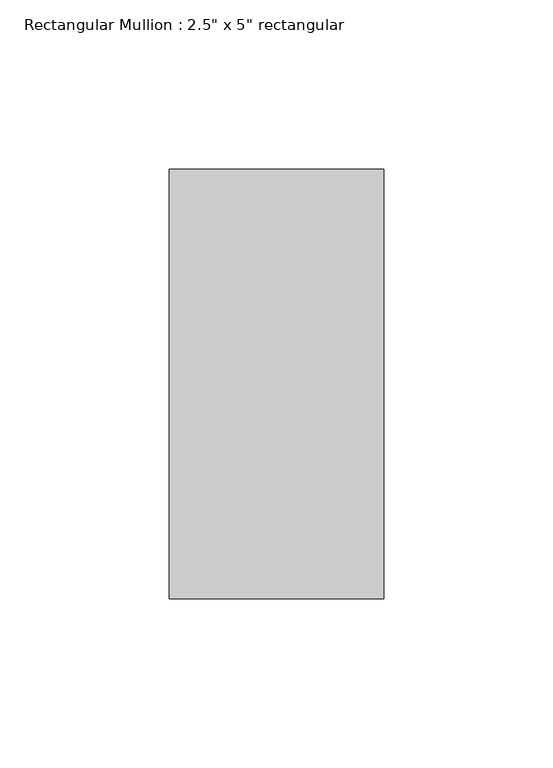
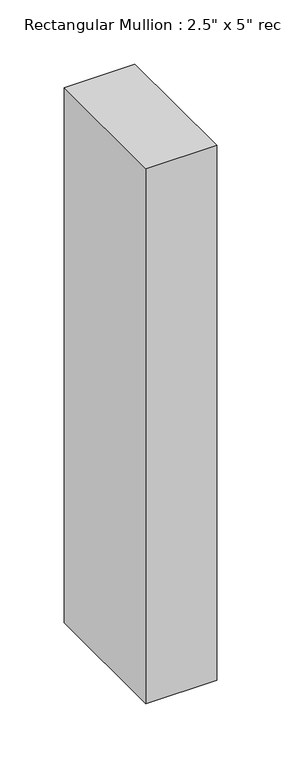
"""IFC4 building model written with IfcOpenShell, lengths in millimetres: member geometry."""

from ifc_helpers import new_model, si_unit, frame, origin, place, context, project, spatial, polyline, outline, extrude, source, transform, mapped, element, save


def member_90750a43(model_context):
    return source(origin(), model_context, "Body", "SweptSolid", [
        extrude(outline(polyline([(31.75, 63.5), (31.75, -63.5), (-31.75, -63.5), (-31.75, 63.5), (31.75, 63.5)])), frame((0.0, 0.0, -508.0), z_axis=(0.0, 0.0, 1.0), x_axis=(1.0, 0.0, 0.0)), (0.0, 0.0, 1.0), 508.0),
    ])


if __name__ == "__main__":
    model = new_model("IFC4")
    model_context = context("Model", 3, world=origin())
    ifc_project = project(units=[si_unit("LENGTHUNIT", "METRE", prefix="MILLI")], contexts=[model_context])
    site = spatial("IfcSite", under=ifc_project)
    building = spatial("IfcBuilding", under=site)
    placement = place(None, origin())
    member_shape = member_90750a43(model_context)
    element("IfcMember", 1, ObjectType="Rectangular Mullion : 2.5\" x 5\" rectangular", at=placement, inside=building, context=model_context, shape_type="MappedRepresentation", body=[
        mapped(member_shape, transform((0.0, 0.0, 0.0), x_axis=(1.0, 0.0, 0.0), y_axis=(0.0, 1.0, 0.0), z_axis=(0.0, 0.0, 1.0))),
    ])
    save(model, "model.ifc")

# Revit data of these elements
# Type "Rectangular Mullion : 2.5\" x 5\" rectangular"
#   built-in parameter 1007304 = 0.416667 (stored number, unit not read)
#   built-in parameter 1007301 = 0.104167 (stored number, unit not read)
#   built-in parameter 1007300 = 0.104167 (stored number, unit not read)
# Element 1 (IfcMember, "Rectangular Mullion : 2.5\" x 5\" rectangular")
#   Materials on its faces: "Aluminum"
# Materials
#   "Aluminum": class "Metal", colour RGB 247 247 247, transparency 0, Description = "Aluminum 6061", Cost = 0
